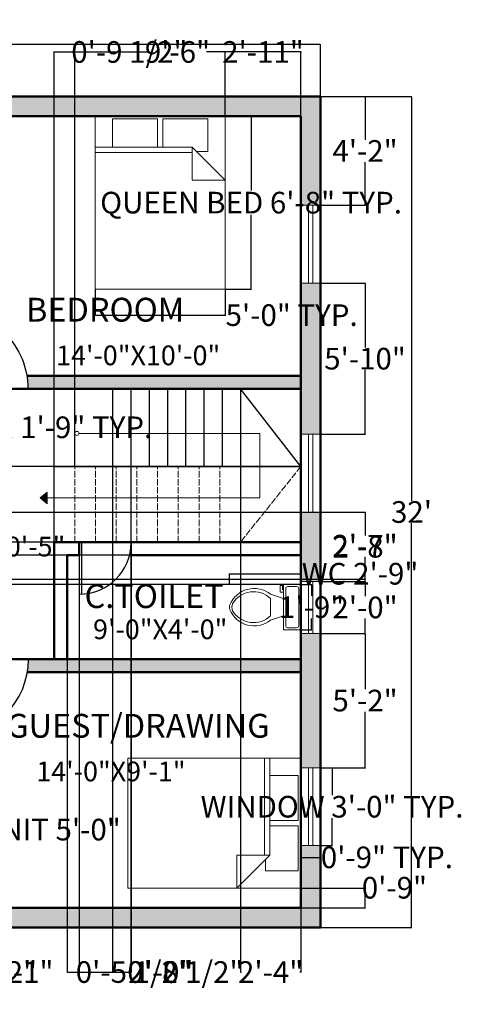
# Model space of a CAD drawing. Units: inches. Extents: x 168 to 640, y -211 to 244.
# Tile 3 of 3: x 436 to 640, y -211 to 244. Entities that reach past the tile are written whole.
import ezdxf

# ---------------------------------------------------------------- set-up
doc = ezdxf.new("R2010")
doc.units = ezdxf.units.IN
doc.header["$MEASUREMENT"] = 0
doc.linetypes.add('ACAD_ISO02W100', pattern=[15, 12, -3])
for name, color, linetype, lineweight in [('A-ANNO-DIMS', 2, 'Continuous', 18), ('A-ANNO-SYMB', 7, 'Continuous', 18), ('A-AREA-IDEN', 7, 'Continuous', 25), ('A-DOOR', 4, 'Continuous', 25), ('A-FLOR-FIXT', 9, 'Continuous', 18), ('A-FLOR-STRS', 7, 'Continuous', 25), ('A-FLOR-STRS-OVHD', 8, 'ACAD_ISO02W100', 18), ('A-FURN', 8, 'Continuous', 18), ('A-GLAZ', 4, 'Continuous', 18), ('A-WALL', 7, 'Continuous', 50)]:
    doc.layers.add(name, color=color, linetype=linetype, lineweight=lineweight)
doc.layers.add('A-WALL-PATT', color=251, linetype='Continuous', lineweight=13, true_color=0x636466)
doc.styles.get("Standard").update_dxf_attribs({"font": 'arial.ttf'})
doc.dimstyles.get("Standard").update_dxf_attribs({"dimtxt": 10, "dimasz": 0.18, "dimexe": 0.18, "dimexo": 0.0625, "dimgap": 0.09, "dimtad": 0, "dimtih": 1, "dimtoh": 1, "dimdec": 0, "dimzin": 0, "dimdsep": 46, "dimlunit": 3, "dimtxsty": 'Standard', "dimcen": 0.09, "dimadec": 0, "dimazin": 0, "dimtfac": 1, "dimtdec": 0, "dimtofl": 0, "dimtmove": 0, "dimatfit": 3, "dimfxl": 1, "dimtolj": 1, "dimtzin": 0, "dimarcsym": 0})

# ---------------------------------------------------------------- blocks, each defined once
blk = doc.blocks.new('*D1')
at = {"layer": 'A-ANNO-DIMS', "color": 0, "lineweight": -2, "transparency": 16777216}
for p, q in [((574.7, 208.8), (616.93, 208.8)), ((616.75, 208.62), (616.75, 22)), ((616.75, -175.02), (616.75, 11.6)), ((574.7, -175.2), (616.93, -175.2))]:
    blk.add_line(p, q, dxfattribs=at)
at = {"layer": 'A-ANNO-DIMS', "color": 0, "transparency": 16777216}
for points in [[(616.72, 208.62), (616.78, 208.62), (616.75, 208.8)], [(616.72, -175.02), (616.78, -175.02), (616.75, -175.2)]]:
    blk.add_solid(points, dxfattribs=at)
at = {"layer": 'Defpoints', "color": 0, "transparency": 16777216}
for p in [(574.63, 208.8), (574.63, -175.2), (616.75, -175.2)]:
    blk.add_point(p, dxfattribs=at)
at = {"layer": 'A-ANNO-DIMS', "color": 0, "transparency": 16777216, "insert": (616.75, 16.8), "char_height": 10, "attachment_point": 5}
blk.add_mtext("\\A1;32'", dxfattribs=at)
blk = doc.blocks.new('*D2')
at = {"layer": 'A-ANNO-DIMS', "color": 0, "lineweight": -2, "transparency": 16777216}
for p, q in [((214.63, 208.86), (214.63, 233.12)), ((214.81, 232.94), (386.06, 232.94)), ((574.45, 232.94), (403.21, 232.94)), ((574.63, 208.86), (574.63, 233.12))]:
    blk.add_line(p, q, dxfattribs=at)
at = {"layer": 'A-ANNO-DIMS', "color": 0, "transparency": 16777216}
for points in [[(214.81, 232.97), (214.81, 232.91), (214.63, 232.94)], [(574.45, 232.97), (574.45, 232.91), (574.63, 232.94)]]:
    blk.add_solid(points, dxfattribs=at)
at = {"layer": 'Defpoints', "color": 0, "transparency": 16777216}
for p in [(214.63, 232.94), (214.63, 208.8), (574.63, 208.8)]:
    blk.add_point(p, dxfattribs=at)
at = {"layer": 'A-ANNO-DIMS', "color": 0, "transparency": 16777216, "insert": (394.63, 232.94), "char_height": 10, "attachment_point": 5}
blk.add_mtext("\\A1;30'", dxfattribs=at)
blk = doc.blocks.new('Toilet - top')
for p, q in [((9.5, -6), (9.5, -2)), ((-10, -8.5), (-8, -8.5)), ((-10, -9.5), (-10, -8.5)), ((-8, -8.5), (-8, -8)), ((-7, -8), (-7, -9.5)), ((-4, -8), (-6, -14)), ((4, -8), (6, -14)), ((-7, -9.5), (-10, -9.5)), ((4, -14), (-4, -14))]:
    blk.add_line(p, q)
blk.add_lwpolyline([(10.5, -8), (10.5, 0), (-10.5, 0), (-10.5, -8)], close=True)
for points in [[(-9.5, -2), (-9.5, -6)], [(8.5, -1), (-8.5, -1)], [(-8.5, -7), (8.5, -7)]]:
    blk.add_lwpolyline(points)
for centre, radius, start, end in [((-8.62, -1.88), 0.884, 81.8699, 188.1301), ((8.62, -1.88), 0.884, 351.8699, 98.1301), ((-8.62, -6.12), 0.884, 171.8699, 278.1301), ((8.62, -6.12), 0.884, 261.8699, 8.1301), ((3.52, -21.58), 12.17, 141.4691, 247.9714), ((4.2, -21.82), 11.33, 136.3677, 238.9468), ((-3.52, -21.58), 12.17, 292.0284, 38.5307), ((-4.2, -21.82), 11.33, 301.053, 43.6321), ((0, -27.88), 4, 245.7318, 294.2682), ((0, -29), 4, 254.8605, 285.1395)]:
    blk.add_arc(centre, radius, start, end)
blk = doc.blocks.new('Bed - Queen')
for p, q in [((0, -80.00003), (0, 0)), ((0, 0), (59.99999, 0)), ((59.99999, 0), (59.99999, -80.00003)), ((7.99999, -1.2), (28.79998, -1.2)), ((7.99999, -14.4), (7.99999, -1.2)), ((28.79998, -1.2), (28.79998, -14.4)), ((31.19999, -1.2), (51.99999, -1.2)), ((31.19999, -14.4), (31.19999, -1.2)), ((51.99999, -1.2), (51.99999, -16.4)), ((0, -14.4), (44.8, -14.4)), ((44.8, -16.8), (0, -16.8)), ((59.99999, -29.6), (44.8, -14.4)), ((44.8, -14.4), (44.8, -29.6)), ((51.99999, -16.4), (46.79936, -16.4)), ((44.8, -29.6), (59.99999, -29.6)), ((59.99999, -80.00003), (0, -80.00003))]:
    blk.add_line(p, q)
blk = doc.blocks.new('DOOR-SWING-36IN')
for p, q in [((0, 36), (0, 0)), ((1, 36), (1, 0))]:
    blk.add_line(p, q)
blk.add_arc((0, 36), 36, 270, 0)
blk = doc.blocks.new('WIN-36IN-WALL9')
at = {"ltscale": 0.25}
for p, q in [((0, 36), (9, 36)), ((3.5, 36), (3.5, 0)), ((5.5, 36), (5.5, 0)), ((9, 0), (0, 0))]:
    blk.add_line(p, q, dxfattribs=at)
blk = doc.blocks.new('*D9')
at = {"layer": 'A-ANNO-DIMS', "color": 0, "lineweight": -2, "ltscale": 0.25, "transparency": 16777216}
for p, q in [((574.7, -101.43), (580.21, -101.43)), ((580.03, -101.61), (580.03, -114.16)), ((580.03, -137.25), (580.03, -124.7)), ((574.7, -137.43), (580.21, -137.43))]:
    blk.add_line(p, q, dxfattribs=at)
at = {"layer": 'A-ANNO-DIMS', "color": 0, "ltscale": 0.25, "transparency": 16777216}
for points in [[(580, -101.61), (580.06, -101.61), (580.03, -101.43)], [(580, -137.25), (580.06, -137.25), (580.03, -137.43)]]:
    blk.add_solid(points, dxfattribs=at)
at = {"layer": 'Defpoints', "color": 0, "ltscale": 0.25, "transparency": 16777216}
for p in [(574.63, -101.43), (580.03, -101.43), (574.63, -137.43)]:
    blk.add_point(p, dxfattribs=at)
at = {"layer": 'A-ANNO-DIMS', "color": 0, "ltscale": 0.25, "transparency": 16777216, "insert": (580.03, -119.43), "char_height": 10, "attachment_point": 5}
blk.add_mtext('\\A1;WINDOW 3\'-0" TYP.', dxfattribs=at)
blk = doc.blocks.new('*D10')
at = {"layer": 'A-ANNO-DIMS', "color": 0, "lineweight": -2, "ltscale": 0.25, "transparency": 16777216}
for p, q in [((565.63, -137.49), (565.63, -143.01)), ((574.63, -137.49), (574.63, -143.01)), ((565.81, -142.83), (574.45, -142.83)), ((574.63, -142.83), (574.81, -142.83))]:
    blk.add_line(p, q, dxfattribs=at)
at = {"layer": 'A-ANNO-DIMS', "color": 0, "ltscale": 0.25, "transparency": 16777216}
for points in [[(565.81, -142.8), (565.81, -142.86), (565.63, -142.83)], [(574.45, -142.8), (574.45, -142.86), (574.63, -142.83)]]:
    blk.add_solid(points, dxfattribs=at)
at = {"layer": 'Defpoints', "color": 0, "ltscale": 0.25, "transparency": 16777216}
for p in [(565.63, -137.43), (574.63, -137.43), (574.63, -142.83)]:
    blk.add_point(p, dxfattribs=at)
at = {"layer": 'A-ANNO-DIMS', "color": 0, "ltscale": 0.25, "transparency": 16777216, "insert": (605.38, -142.83), "char_height": 10, "attachment_point": 5}
blk.add_mtext('\\A1;0\'-9" TYP.', dxfattribs=at)
blk = doc.blocks.new('*D13')
at = {"layer": 'A-ANNO-DIMS', "color": 0, "lineweight": -2, "ltscale": 0.25, "transparency": 16777216}
for p, q in [((530.7, 199.8), (542.82, 199.8)), ((542.64, 199.62), (542.64, 165.37)), ((542.64, 119.98), (542.64, 154.23)), ((530.7, 119.8), (542.82, 119.8))]:
    blk.add_line(p, q, dxfattribs=at)
at = {"layer": 'A-ANNO-DIMS', "color": 0, "ltscale": 0.25, "transparency": 16777216}
for points in [[(542.61, 199.62), (542.67, 199.62), (542.64, 199.8)], [(542.61, 119.98), (542.67, 119.98), (542.64, 119.8)]]:
    blk.add_solid(points, dxfattribs=at)
at = {"layer": 'Defpoints', "color": 0, "ltscale": 0.25, "transparency": 16777216}
for p in [(530.64, 199.8), (542.64, 199.8), (530.64, 119.8)]:
    blk.add_point(p, dxfattribs=at)
at = {"layer": 'A-ANNO-DIMS', "color": 0, "ltscale": 0.25, "transparency": 16777216, "insert": (542.64, 159.8), "char_height": 10, "attachment_point": 5}
blk.add_mtext('\\A1;QUEEN BED 6\'-8" TYP.', dxfattribs=at)
blk = doc.blocks.new('*D14')
at = {"layer": 'A-ANNO-DIMS', "color": 0, "lineweight": -2, "ltscale": 0.25, "transparency": 16777216}
for p, q in [((470.64, 119.74), (470.64, 107.62)), ((530.64, 119.74), (530.64, 107.62)), ((470.82, 107.8), (530.46, 107.8)), ((530.64, 107.8), (530.82, 107.8))]:
    blk.add_line(p, q, dxfattribs=at)
at = {"layer": 'A-ANNO-DIMS', "color": 0, "ltscale": 0.25, "transparency": 16777216}
for points in [[(470.82, 107.83), (470.82, 107.77), (470.64, 107.8)], [(530.46, 107.83), (530.46, 107.77), (530.64, 107.8)]]:
    blk.add_solid(points, dxfattribs=at)
at = {"layer": 'Defpoints', "color": 0, "ltscale": 0.25, "transparency": 16777216}
for p in [(470.64, 119.8), (530.64, 119.8), (530.64, 107.8)]:
    blk.add_point(p, dxfattribs=at)
at = {"layer": 'A-ANNO-DIMS', "color": 0, "ltscale": 0.25, "transparency": 16777216, "insert": (561.38, 107.8), "char_height": 10, "attachment_point": 5}
blk.add_mtext('\\A1;5\'-0" TYP.', dxfattribs=at)
blk = doc.blocks.new('*D15')
at = {"layer": 'A-ANNO-DIMS', "color": 0, "lineweight": -2, "ltscale": 0.25, "transparency": 16777216}
for p, q in [((318.79, 52.86), (318.79, 56.13)), ((318.97, 55.95), (339.61, 55.95)), ((339.79, 52.86), (339.79, 56.13)), ((339.79, 55.95), (339.97, 55.95))]:
    blk.add_line(p, q, dxfattribs=at)
at = {"layer": 'A-ANNO-DIMS', "color": 0, "ltscale": 0.25, "transparency": 16777216}
for points in [[(318.97, 55.98), (318.97, 55.92), (318.79, 55.95)], [(339.61, 55.98), (339.61, 55.92), (339.79, 55.95)]]:
    blk.add_solid(points, dxfattribs=at)
at = {"layer": 'Defpoints', "color": 0, "ltscale": 0.25, "transparency": 16777216}
for p in [(339.79, 55.95), (318.79, 52.8), (339.79, 52.8)]:
    blk.add_point(p, dxfattribs=at)
at = {"layer": 'A-ANNO-DIMS', "color": 0, "ltscale": 0.25, "transparency": 16777216, "insert": (420.35, 55.95), "char_height": 10, "attachment_point": 5}
blk.add_mtext('\\A1;DINING CHAIR 1\'-9" TYP.', dxfattribs=at)
blk = doc.blocks.new('*D17')
at = {"layer": 'A-ANNO-DIMS', "color": 0, "lineweight": -2, "ltscale": 0.25, "transparency": 16777216}
for p, q in [((532.59, -16.64), (532.59, -11.56)), ((532.77, -11.74), (565.45, -11.74)), ((565.63, -16.64), (565.63, -11.56)), ((565.63, -11.74), (565.81, -11.74))]:
    blk.add_line(p, q, dxfattribs=at)
at = {"layer": 'A-ANNO-DIMS', "color": 0, "ltscale": 0.25, "transparency": 16777216}
for points in [[(532.77, -11.71), (532.77, -11.77), (532.59, -11.74)], [(565.45, -11.71), (565.45, -11.77), (565.63, -11.74)]]:
    blk.add_solid(points, dxfattribs=at)
at = {"layer": 'Defpoints', "color": 0, "ltscale": 0.25, "transparency": 16777216}
for p in [(565.63, -11.74), (532.59, -16.7), (565.63, -16.7)]:
    blk.add_point(p, dxfattribs=at)
at = {"layer": 'A-ANNO-DIMS', "color": 0, "ltscale": 0.25, "transparency": 16777216, "insert": (592.98, -11.74), "char_height": 10, "attachment_point": 5}
blk.add_mtext('\\A1;WC 2\'-9"', dxfattribs=at)
blk = doc.blocks.new('*D18')
at = {"layer": 'A-ANNO-DIMS', "color": 0, "lineweight": -2, "ltscale": 0.25, "transparency": 16777216}
for p, q in [((565.7, -16.7), (570.77, -16.7)), ((570.59, -16.88), (570.59, -22)), ((570.59, -37.52), (570.59, -32.4)), ((565.7, -37.7), (570.77, -37.7))]:
    blk.add_line(p, q, dxfattribs=at)
at = {"layer": 'A-ANNO-DIMS', "color": 0, "ltscale": 0.25, "transparency": 16777216}
for points in [[(570.56, -16.88), (570.62, -16.88), (570.59, -16.7)], [(570.56, -37.52), (570.62, -37.52), (570.59, -37.7)]]:
    blk.add_solid(points, dxfattribs=at)
at = {"layer": 'Defpoints', "color": 0, "ltscale": 0.25, "transparency": 16777216}
for p in [(565.63, -16.7), (565.63, -37.7), (570.59, -37.7)]:
    blk.add_point(p, dxfattribs=at)
at = {"layer": 'A-ANNO-DIMS', "color": 0, "ltscale": 0.25, "transparency": 16777216, "insert": (570.59, -27.2), "char_height": 10, "attachment_point": 5}
blk.add_mtext('\\A1;1\'-9"', dxfattribs=at)
blk = doc.blocks.new('*D19')
at = {"layer": 'A-ANNO-DIMS', "color": 0, "lineweight": -2, "ltscale": 0.25, "transparency": 16777216}
for p, q in [((419.03, -100), (428.15, -100)), ((427.97, -100.18), (427.97, -124.81)), ((427.97, -159.82), (427.97, -135.2)), ((419.03, -160), (428.15, -160))]:
    blk.add_line(p, q, dxfattribs=at)
at = {"layer": 'A-ANNO-DIMS', "color": 0, "ltscale": 0.25, "transparency": 16777216}
for points in [[(427.94, -100.18), (428, -100.18), (427.97, -100)], [(427.94, -159.82), (428, -159.82), (427.97, -160)]]:
    blk.add_solid(points, dxfattribs=at)
at = {"layer": 'Defpoints', "color": 0, "ltscale": 0.25, "transparency": 16777216}
for p in [(418.97, -100), (427.97, -100), (418.97, -160)]:
    blk.add_point(p, dxfattribs=at)
at = {"layer": 'A-ANNO-DIMS', "color": 0, "ltscale": 0.25, "transparency": 16777216, "insert": (427.97, -130), "char_height": 10, "attachment_point": 5}
blk.add_mtext('\\A1;MEDIA UNIT 5\'-0"', dxfattribs=at)
blk = doc.blocks.new('*D23')
at = {"layer": 'A-ANNO-DIMS', "color": 0, "lineweight": -2, "ltscale": 0.25, "transparency": 16777216}
for p, q in [((574.7, 208.8), (595.46, 208.8)), ((595.28, 208.62), (595.28, 188.79)), ((595.28, 158.75), (595.28, 178.57)), ((574.7, 158.57), (595.46, 158.57))]:
    blk.add_line(p, q, dxfattribs=at)
at = {"layer": 'A-ANNO-DIMS', "color": 0, "ltscale": 0.25, "transparency": 16777216}
for points in [[(595.25, 208.62), (595.31, 208.62), (595.28, 208.8)], [(595.25, 158.75), (595.31, 158.75), (595.28, 158.57)]]:
    blk.add_solid(points, dxfattribs=at)
at = {"layer": 'Defpoints', "color": 0, "ltscale": 0.25, "transparency": 16777216}
for p in [(574.63, 208.8), (574.63, 158.57), (595.28, 158.57)]:
    blk.add_point(p, dxfattribs=at)
at = {"layer": 'A-ANNO-DIMS', "color": 0, "ltscale": 0.25, "transparency": 16777216, "insert": (595.28, 183.68), "char_height": 10, "attachment_point": 5}
blk.add_mtext('\\A1;4\'-2"', dxfattribs=at)
blk = doc.blocks.new('*D24')
at = {"layer": 'A-ANNO-DIMS', "color": 0, "lineweight": -2, "ltscale": 0.25, "transparency": 16777216}
for p, q in [((574.7, 122.57), (595.46, 122.57)), ((595.28, 122.39), (595.28, 92.88)), ((595.28, 52.98), (595.28, 82.49)), ((574.7, 52.8), (595.46, 52.8))]:
    blk.add_line(p, q, dxfattribs=at)
at = {"layer": 'A-ANNO-DIMS', "color": 0, "ltscale": 0.25, "transparency": 16777216}
for points in [[(595.25, 122.39), (595.31, 122.39), (595.28, 122.57)], [(595.25, 52.98), (595.31, 52.98), (595.28, 52.8)]]:
    blk.add_solid(points, dxfattribs=at)
at = {"layer": 'Defpoints', "color": 0, "ltscale": 0.25, "transparency": 16777216}
for p in [(574.63, 122.57), (574.63, 52.8), (595.28, 52.8)]:
    blk.add_point(p, dxfattribs=at)
at = {"layer": 'A-ANNO-DIMS', "color": 0, "ltscale": 0.25, "transparency": 16777216, "insert": (595.28, 87.68), "char_height": 10, "attachment_point": 5}
blk.add_mtext('\\A1;5\'-10"', dxfattribs=at)
blk = doc.blocks.new('*D25')
at = {"layer": 'A-ANNO-DIMS', "color": 0, "lineweight": -2, "ltscale": 0.25, "transparency": 16777216}
for p, q in [((574.7, 16.8), (595.46, 16.8)), ((595.28, 16.62), (595.28, 5.93)), ((595.28, -15.15), (595.28, -4.46)), ((574.7, -15.33), (595.46, -15.33))]:
    blk.add_line(p, q, dxfattribs=at)
at = {"layer": 'A-ANNO-DIMS', "color": 0, "ltscale": 0.25, "transparency": 16777216}
for points in [[(595.25, 16.62), (595.31, 16.62), (595.28, 16.8)], [(595.25, -15.15), (595.31, -15.15), (595.28, -15.33)]]:
    blk.add_solid(points, dxfattribs=at)
at = {"layer": 'Defpoints', "color": 0, "ltscale": 0.25, "transparency": 16777216}
for p in [(574.63, 16.8), (574.63, -15.33), (595.28, -15.33)]:
    blk.add_point(p, dxfattribs=at)
at = {"layer": 'A-ANNO-DIMS', "color": 0, "ltscale": 0.25, "transparency": 16777216, "insert": (595.28, 0.74), "char_height": 10, "attachment_point": 5}
blk.add_mtext('\\A1;2\'-8"', dxfattribs=at)
blk = doc.blocks.new('*D26')
at = {"layer": 'A-ANNO-DIMS', "color": 0, "lineweight": -2, "ltscale": 0.25, "transparency": 16777216}
for p, q in [((574.7, -15.33), (595.46, -15.33)), ((595.28, -15.51), (595.28, -22.11)), ((595.28, -39.11), (595.28, -32.5)), ((574.7, -39.29), (595.46, -39.29))]:
    blk.add_line(p, q, dxfattribs=at)
at = {"layer": 'A-ANNO-DIMS', "color": 0, "ltscale": 0.25, "transparency": 16777216}
for points in [[(595.25, -15.51), (595.31, -15.51), (595.28, -15.33)], [(595.25, -39.11), (595.31, -39.11), (595.28, -39.29)]]:
    blk.add_solid(points, dxfattribs=at)
at = {"layer": 'Defpoints', "color": 0, "ltscale": 0.25, "transparency": 16777216}
for p in [(574.63, -15.33), (574.63, -39.29), (595.28, -39.29)]:
    blk.add_point(p, dxfattribs=at)
at = {"layer": 'A-ANNO-DIMS', "color": 0, "ltscale": 0.25, "transparency": 16777216, "insert": (595.28, -27.31), "char_height": 10, "attachment_point": 5}
blk.add_mtext('\\A1;2\'-0"', dxfattribs=at)
blk = doc.blocks.new('*D27')
at = {"layer": 'A-ANNO-DIMS', "color": 0, "lineweight": -2, "ltscale": 0.25, "transparency": 16777216}
for p, q in [((574.7, -39.29), (595.46, -39.29)), ((595.28, -39.47), (595.28, -65.16)), ((595.28, -101.25), (595.28, -75.56)), ((574.7, -101.43), (595.46, -101.43))]:
    blk.add_line(p, q, dxfattribs=at)
at = {"layer": 'A-ANNO-DIMS', "color": 0, "ltscale": 0.25, "transparency": 16777216}
for points in [[(595.25, -39.47), (595.31, -39.47), (595.28, -39.29)], [(595.25, -101.25), (595.31, -101.25), (595.28, -101.43)]]:
    blk.add_solid(points, dxfattribs=at)
at = {"layer": 'Defpoints', "color": 0, "ltscale": 0.25, "transparency": 16777216}
for p in [(574.63, -39.29), (574.63, -101.43), (595.28, -101.43)]:
    blk.add_point(p, dxfattribs=at)
at = {"layer": 'A-ANNO-DIMS', "color": 0, "ltscale": 0.25, "transparency": 16777216, "insert": (595.28, -70.36), "char_height": 10, "attachment_point": 5}
blk.add_mtext('\\A1;5\'-2"', dxfattribs=at)
blk = doc.blocks.new('*D32')
at = {"layer": 'A-ANNO-DIMS', "color": 0, "lineweight": -2, "ltscale": 0.25, "transparency": 16777216}
for p, q in [((451.63, 2.86), (451.63, 229.63)), ((451.81, 229.45), (495.25, 229.45)), ((565.45, 229.45), (522.02, 229.45)), ((565.63, 2.86), (565.63, 229.63))]:
    blk.add_line(p, q, dxfattribs=at)
at = {"layer": 'A-ANNO-DIMS', "color": 0, "ltscale": 0.25, "transparency": 16777216}
for points in [[(451.81, 229.48), (451.81, 229.42), (451.63, 229.45)], [(565.45, 229.48), (565.45, 229.42), (565.63, 229.45)]]:
    blk.add_solid(points, dxfattribs=at)
at = {"layer": 'Defpoints', "color": 0, "ltscale": 0.25, "transparency": 16777216}
for p in [(565.63, 229.45), (451.63, 2.8), (565.63, 2.8)]:
    blk.add_point(p, dxfattribs=at)
at = {"layer": 'A-ANNO-DIMS', "color": 0, "ltscale": 0.25, "transparency": 16777216, "insert": (508.63, 229.45), "char_height": 10, "attachment_point": 5}
blk.add_mtext('\\A1;9\'-6"', dxfattribs=at)
blk = doc.blocks.new('*D33')
at = {"layer": 'A-ANNO-DIMS', "color": 0, "lineweight": -2, "ltscale": 0.25, "transparency": 16777216}
for p, q in [((565.57, 73.8), (193.8, 73.8)), ((193.98, 73.62), (193.98, 61)), ((193.98, 37.98), (193.98, 50.6)), ((565.57, 37.8), (193.8, 37.8))]:
    blk.add_line(p, q, dxfattribs=at)
at = {"layer": 'A-ANNO-DIMS', "color": 0, "ltscale": 0.25, "transparency": 16777216}
for points in [[(193.95, 73.62), (194.01, 73.62), (193.98, 73.8)], [(193.95, 37.98), (194.01, 37.98), (193.98, 37.8)]]:
    blk.add_solid(points, dxfattribs=at)
at = {"layer": 'Defpoints', "color": 0, "ltscale": 0.25, "transparency": 16777216}
for p in [(193.98, 73.8), (565.63, 73.8), (565.63, 37.8)]:
    blk.add_point(p, dxfattribs=at)
at = {"layer": 'A-ANNO-DIMS', "color": 0, "ltscale": 0.25, "transparency": 16777216, "insert": (193.98, 55.8), "char_height": 10, "attachment_point": 5}
blk.add_mtext('\\A1;3\'-0"', dxfattribs=at)
blk = doc.blocks.new('*D34')
at = {"layer": 'A-ANNO-DIMS', "color": 0, "lineweight": -2, "ltscale": 0.25, "transparency": 16777216}
for p, q in [((451.57, 37.8), (193.8, 37.8)), ((193.98, 37.62), (193.98, 25.41)), ((193.98, 2.98), (193.98, 15.19)), ((451.57, 2.8), (193.8, 2.8))]:
    blk.add_line(p, q, dxfattribs=at)
at = {"layer": 'A-ANNO-DIMS', "color": 0, "ltscale": 0.25, "transparency": 16777216}
for points in [[(193.95, 37.62), (194.01, 37.62), (193.98, 37.8)], [(193.95, 2.98), (194.01, 2.98), (193.98, 2.8)]]:
    blk.add_solid(points, dxfattribs=at)
at = {"layer": 'Defpoints', "color": 0, "ltscale": 0.25, "transparency": 16777216}
for p in [(193.98, 37.8), (451.63, 37.8), (451.63, 2.8)]:
    blk.add_point(p, dxfattribs=at)
at = {"layer": 'A-ANNO-DIMS', "color": 0, "ltscale": 0.25, "transparency": 16777216, "insert": (193.98, 20.3), "char_height": 10, "attachment_point": 5}
blk.add_mtext('\\A1;2\'-11"', dxfattribs=at)
blk = doc.blocks.new('*D40')
at = {"layer": 'A-ANNO-DIMS', "color": 0, "lineweight": -2, "ltscale": 0.25, "transparency": 16777216}
for p, q in [((457.63, -3.26), (457.63, -196.03)), ((463.26, -3.26), (463.26, -196.03)), ((457.81, -195.85), (463.08, -195.85)), ((463.26, -195.85), (463.44, -195.85))]:
    blk.add_line(p, q, dxfattribs=at)
at = {"layer": 'A-ANNO-DIMS', "color": 0, "ltscale": 0.25, "transparency": 16777216}
for points in [[(457.81, -195.82), (457.81, -195.88), (457.63, -195.85)], [(463.08, -195.82), (463.08, -195.88), (463.26, -195.85)]]:
    blk.add_solid(points, dxfattribs=at)
at = {"layer": 'Defpoints', "color": 0, "ltscale": 0.25, "transparency": 16777216}
for p in [(457.63, -3.2), (463.26, -3.2), (463.26, -195.85)]:
    blk.add_point(p, dxfattribs=at)
at = {"layer": 'A-ANNO-DIMS', "color": 0, "ltscale": 0.25, "transparency": 16777216, "insert": (488.48, -195.85), "char_height": 10, "attachment_point": 5}
blk.add_mtext('\\A1;0\'-5 1/2"', dxfattribs=at)
blk = doc.blocks.new('*D41')
at = {"layer": 'A-ANNO-DIMS', "color": 0, "lineweight": -2, "ltscale": 0.25, "transparency": 16777216}
for p, q in [((463.26, 2.74), (463.26, -196.03)), ((487.26, 2.74), (487.26, -196.03)), ((463.44, -195.85), (487.08, -195.85)), ((487.26, -195.85), (487.44, -195.85))]:
    blk.add_line(p, q, dxfattribs=at)
at = {"layer": 'A-ANNO-DIMS', "color": 0, "ltscale": 0.25, "transparency": 16777216}
for points in [[(463.44, -195.82), (463.44, -195.88), (463.26, -195.85)], [(487.08, -195.82), (487.08, -195.88), (487.26, -195.85)]]:
    blk.add_solid(points, dxfattribs=at)
at = {"layer": 'Defpoints', "color": 0, "ltscale": 0.25, "transparency": 16777216}
for p in [(463.26, 2.8), (487.26, 2.8), (487.26, -195.85)]:
    blk.add_point(p, dxfattribs=at)
at = {"layer": 'A-ANNO-DIMS', "color": 0, "ltscale": 0.25, "transparency": 16777216, "insert": (500.91, -195.85), "char_height": 10, "attachment_point": 5}
blk.add_mtext('\\A1;2\'-0"', dxfattribs=at)
blk = doc.blocks.new('*D42')
at = {"layer": 'A-ANNO-DIMS', "color": 0, "lineweight": -2, "ltscale": 0.25, "transparency": 16777216}
for p, q in [((537.7, 37.74), (537.7, -196.03)), ((565.63, 37.74), (565.63, -196.03)), ((537.88, -195.85), (538.2, -195.85)), ((565.45, -195.85), (565.14, -195.85))]:
    blk.add_line(p, q, dxfattribs=at)
at = {"layer": 'A-ANNO-DIMS', "color": 0, "ltscale": 0.25, "transparency": 16777216}
for points in [[(537.88, -195.82), (537.88, -195.88), (537.7, -195.85)], [(565.45, -195.82), (565.45, -195.88), (565.63, -195.85)]]:
    blk.add_solid(points, dxfattribs=at)
at = {"layer": 'Defpoints', "color": 0, "ltscale": 0.25, "transparency": 16777216}
for p in [(537.7, 37.8), (565.63, 37.8), (565.63, -195.85)]:
    blk.add_point(p, dxfattribs=at)
at = {"layer": 'A-ANNO-DIMS', "color": 0, "ltscale": 0.25, "transparency": 16777216, "insert": (551.67, -195.85), "char_height": 10, "attachment_point": 5}
blk.add_mtext('\\A1;2\'-4"', dxfattribs=at)
blk = doc.blocks.new('*D43')
at = {"layer": 'A-ANNO-DIMS', "color": 0, "lineweight": -2, "ltscale": 0.25, "transparency": 16777216}
for p, q in [((478.63, 73.74), (478.63, -196.03)), ((487.07, 73.74), (487.07, -196.03)), ((478.81, -195.85), (486.89, -195.85)), ((487.07, -195.85), (487.25, -195.85))]:
    blk.add_line(p, q, dxfattribs=at)
at = {"layer": 'A-ANNO-DIMS', "color": 0, "ltscale": 0.25, "transparency": 16777216}
for points in [[(478.81, -195.82), (478.81, -195.88), (478.63, -195.85)], [(486.89, -195.82), (486.89, -195.88), (487.07, -195.85)]]:
    blk.add_solid(points, dxfattribs=at)
at = {"layer": 'Defpoints', "color": 0, "ltscale": 0.25, "transparency": 16777216}
for p in [(478.63, 73.8), (487.07, 73.8), (487.07, -195.85)]:
    blk.add_point(p, dxfattribs=at)
at = {"layer": 'A-ANNO-DIMS', "color": 0, "ltscale": 0.25, "transparency": 16777216, "insert": (512.28, -195.85), "char_height": 10, "attachment_point": 5}
blk.add_mtext('\\A1;0\'-8 1/2"', dxfattribs=at)
blk = doc.blocks.new('*D44')
at = {"layer": 'A-ANNO-DIMS', "color": 0, "lineweight": -2, "ltscale": 0.25, "transparency": 16777216}
for p, q in [((451.63, 37.86), (451.63, 229.63)), ((451.81, 229.45), (461.02, 229.45)), ((461.2, 37.86), (461.2, 229.63)), ((461.2, 229.45), (461.38, 229.45))]:
    blk.add_line(p, q, dxfattribs=at)
at = {"layer": 'A-ANNO-DIMS', "color": 0, "ltscale": 0.25, "transparency": 16777216}
for points in [[(451.81, 229.48), (451.81, 229.42), (451.63, 229.45)], [(461.02, 229.48), (461.02, 229.42), (461.2, 229.45)]]:
    blk.add_solid(points, dxfattribs=at)
at = {"layer": 'Defpoints', "color": 0, "ltscale": 0.25, "transparency": 16777216}
for p in [(461.2, 229.45), (451.63, 37.8), (461.2, 37.8)]:
    blk.add_point(p, dxfattribs=at)
at = {"layer": 'A-ANNO-DIMS', "color": 0, "ltscale": 0.25, "transparency": 16777216, "insert": (486.41, 229.45), "char_height": 10, "attachment_point": 5}
blk.add_mtext('\\A1;0\'-9 1/2"', dxfattribs=at)
blk = doc.blocks.new('*D49')
at = {"layer": 'A-ANNO-DIMS', "color": 0, "lineweight": -2, "ltscale": 0.25, "transparency": 16777216}
for p, q in [((252.23, 16.8), (595.46, 16.8)), ((595.28, 16.62), (595.28, 6.35)), ((595.28, -14.14), (595.28, -3.87)), ((252.23, -14.32), (595.46, -14.32))]:
    blk.add_line(p, q, dxfattribs=at)
at = {"layer": 'A-ANNO-DIMS', "color": 0, "ltscale": 0.25, "transparency": 16777216}
for points in [[(595.25, 16.62), (595.31, 16.62), (595.28, 16.8)], [(595.25, -14.14), (595.31, -14.14), (595.28, -14.32)]]:
    blk.add_solid(points, dxfattribs=at)
at = {"layer": 'Defpoints', "color": 0, "ltscale": 0.25, "transparency": 16777216}
for p in [(252.17, 16.8), (595.28, 16.8), (252.17, -14.32)]:
    blk.add_point(p, dxfattribs=at)
at = {"layer": 'A-ANNO-DIMS', "color": 0, "ltscale": 0.25, "transparency": 16777216, "insert": (595.28, 1.24), "char_height": 10, "attachment_point": 5}
blk.add_mtext('\\A1;2\'-7"', dxfattribs=at)
blk = doc.blocks.new('*D53')
at = {"layer": 'A-ANNO-DIMS', "color": 0, "lineweight": -2, "ltscale": 0.25, "transparency": 16777216}
for p, q in [((367.04, 124.86), (367.04, -196.03)), ((391.63, 124.86), (391.63, -196.03)), ((367.22, -195.85), (391.45, -195.85)), ((391.63, -195.85), (391.81, -195.85))]:
    blk.add_line(p, q, dxfattribs=at)
at = {"layer": 'A-ANNO-DIMS', "color": 0, "ltscale": 0.25, "transparency": 16777216}
for points in [[(367.22, -195.82), (367.22, -195.88), (367.04, -195.85)], [(391.45, -195.82), (391.45, -195.88), (391.63, -195.85)]]:
    blk.add_solid(points, dxfattribs=at)
at = {"layer": 'Defpoints', "color": 0, "ltscale": 0.25, "transparency": 16777216}
for p in [(367.04, 124.92), (391.63, 124.92), (391.63, -195.85)]:
    blk.add_point(p, dxfattribs=at)
at = {"layer": 'A-ANNO-DIMS', "color": 0, "ltscale": 0.25, "transparency": 16777216, "insert": (416.93, -195.85), "char_height": 10, "attachment_point": 5}
blk.add_mtext('\\A1;2\'-0 1/2"', dxfattribs=at)
blk = doc.blocks.new('*D55')
at = {"layer": 'A-ANNO-DIMS', "color": 0, "lineweight": -2, "ltscale": 0.25, "transparency": 16777216}
for p, q in [((397.63, 124.86), (397.63, -196.03)), ((422.63, 124.86), (422.63, -196.03)), ((397.81, -195.85), (422.45, -195.85)), ((422.63, -195.85), (422.81, -195.85))]:
    blk.add_line(p, q, dxfattribs=at)
at = {"layer": 'A-ANNO-DIMS', "color": 0, "ltscale": 0.25, "transparency": 16777216}
for points in [[(397.81, -195.82), (397.81, -195.88), (397.63, -195.85)], [(422.45, -195.82), (422.45, -195.88), (422.63, -195.85)]]:
    blk.add_solid(points, dxfattribs=at)
at = {"layer": 'Defpoints', "color": 0, "ltscale": 0.25, "transparency": 16777216}
for p in [(397.63, 124.92), (422.63, 124.92), (422.63, -195.85)]:
    blk.add_point(p, dxfattribs=at)
at = {"layer": 'A-ANNO-DIMS', "color": 0, "ltscale": 0.25, "transparency": 16777216, "insert": (436.28, -195.85), "char_height": 10, "attachment_point": 5}
blk.add_mtext('\\A1;2\'-1"', dxfattribs=at)
blk = doc.blocks.new('*D57')
at = {"layer": 'A-ANNO-DIMS', "color": 0, "lineweight": -2, "ltscale": 0.25, "transparency": 16777216}
for p, q in [((530.46, 229.45), (530.28, 229.45)), ((530.64, 199.86), (530.64, 229.63)), ((565.63, 199.86), (565.63, 229.63)), ((565.81, 229.45), (565.99, 229.45))]:
    blk.add_line(p, q, dxfattribs=at)
at = {"layer": 'A-ANNO-DIMS', "color": 0, "ltscale": 0.25, "transparency": 16777216}
for points in [[(530.46, 229.48), (530.46, 229.42), (530.64, 229.45)], [(565.81, 229.48), (565.81, 229.42), (565.63, 229.45)]]:
    blk.add_solid(points, dxfattribs=at)
at = {"layer": 'Defpoints', "color": 0, "ltscale": 0.25, "transparency": 16777216}
for p in [(565.63, 229.45), (530.64, 199.8), (565.63, 199.8)]:
    blk.add_point(p, dxfattribs=at)
at = {"layer": 'A-ANNO-DIMS', "color": 0, "ltscale": 0.25, "transparency": 16777216, "insert": (548.14, 229.45), "char_height": 10, "attachment_point": 5}
blk.add_mtext('\\A1;2\'-11"', dxfattribs=at)
blk = doc.blocks.new('*D58')
at = {"layer": 'A-ANNO-DIMS', "color": 0, "lineweight": -2, "ltscale": 0.25, "transparency": 16777216}
for p, q in [((565.7, -157.06), (595.46, -157.06)), ((595.28, -157.06), (595.28, -156.88)), ((595.28, -156.88), (595.46, -156.88)), ((595.28, -166.02), (595.28, -157.24)), ((565.7, -166.2), (595.46, -166.2))]:
    blk.add_line(p, q, dxfattribs=at)
at = {"layer": 'A-ANNO-DIMS', "color": 0, "ltscale": 0.25, "transparency": 16777216}
for points in [[(595.25, -157.24), (595.31, -157.24), (595.28, -157.06)], [(595.25, -166.02), (595.31, -166.02), (595.28, -166.2)]]:
    blk.add_solid(points, dxfattribs=at)
at = {"layer": 'Defpoints', "color": 0, "ltscale": 0.25, "transparency": 16777216}
for p in [(565.63, -157.06), (595.28, -157.06), (565.63, -166.2)]:
    blk.add_point(p, dxfattribs=at)
at = {"layer": 'A-ANNO-DIMS', "color": 0, "ltscale": 0.25, "transparency": 16777216, "insert": (608.85, -156.88), "char_height": 10, "attachment_point": 5}
blk.add_mtext('\\A1;0\'-9"', dxfattribs=at)
blk = doc.blocks.new('*D62')
at = {"layer": 'A-ANNO-DIMS', "color": 0, "lineweight": -2, "ltscale": 0.25, "transparency": 16777216}
for p, q in [((565.57, -3.2), (193.8, -3.2)), ((193.98, -3.38), (193.98, -4.69)), ((565.57, -16.7), (193.8, -16.7)), ((193.98, -16.52), (193.98, -15.21))]:
    blk.add_line(p, q, dxfattribs=at)
at = {"layer": 'A-ANNO-DIMS', "color": 0, "ltscale": 0.25, "transparency": 16777216}
for points in [[(193.95, -3.38), (194.01, -3.38), (193.98, -3.2)], [(193.95, -16.52), (194.01, -16.52), (193.98, -16.7)]]:
    blk.add_solid(points, dxfattribs=at)
at = {"layer": 'Defpoints', "color": 0, "ltscale": 0.25, "transparency": 16777216}
for p in [(565.63, -3.2), (193.98, -16.7), (565.63, -16.7)]:
    blk.add_point(p, dxfattribs=at)
at = {"layer": 'A-ANNO-DIMS', "color": 0, "ltscale": 0.25, "transparency": 16777216, "insert": (193.98, -9.95), "char_height": 10, "attachment_point": 5}
blk.add_mtext('\\A1;1\'-1 1/2"', dxfattribs=at)

msp = doc.modelspace()

# ---------------------------------------------------------------- hatches: boundary and pattern name
at = {"layer": 'A-ANNO-SYMB', "ltscale": 0.25}
h = msp.add_hatch(color=256, dxfattribs=at)
h.dxf.hatch_style = 1
h.paths.add_polyline_path([(448.5, 26.03), (445.23, 23.32), (448.5, 23.32)])
h.paths.add_polyline_path([(448.5, 23.32), (445.23, 23.32), (448.5, 20.61)])
at = {"layer": 'A-WALL-PATT', "ltscale": 0.25}
h = msp.add_hatch(color=256, dxfattribs=at)
h.dxf.hatch_style = 1
h.paths.add_polyline_path([(223.63, 11.3), (214.63, 11.3), (214.63, -175.2), (574.63, -175.2), (574.63, -137.43), (565.63, -137.43), (565.63, -157.06), (565.63, -166.2), (223.63, -166.2)])
h.paths.add_polyline_path([(349.62, -51.2), (301.63, -51.2), (223.63, -51.2), (223.63, -57.2), (301.63, -57.2), (349.12, -57.2, -0.041886)], flags=17)
h.paths.add_polyline_path([(301.63, -48.03), (295.63, -48.03), (295.63, -51.2), (301.63, -51.2)], flags=17)
h.paths.add_polyline_path([(403.8, -51.2), (385.12, -51.2), (385.12, -57.2), (403.8, -57.2)], flags=17)
h.paths.add_polyline_path([(397.63, -57.2), (390.63, -57.2), (390.63, -166.2), (397.63, -166.2)], flags=17)
h.paths.add_polyline_path([(301.63, 73.8), (295.63, 73.8), (295.63, -12.53, -0.041886), (301.63, -12.03)])
h.paths.add_polyline_path([(223.63, 122.57), (214.63, 122.57), (214.63, 47.3), (223.63, 47.3), (223.63, 73.8)])
h.paths.add_polyline_path([(350.92, 79.8), (223.63, 79.8), (223.63, 73.8), (350.42, 73.8, -0.041886)])
h.paths.add_polyline_path([(574.63, 208.8), (214.63, 208.8), (214.63, 158.57), (223.63, 158.57), (223.63, 199.8), (565.63, 199.8), (565.63, 158.57), (574.63, 158.57)])
h.paths.add_polyline_path([(397.63, 199.8), (391.63, 199.8), (391.63, 79.8), (386.42, 79.8), (386.42, 73.8), (391.63, 73.8), (403.56, 73.8), (403.56, 79.8), (397.63, 79.8)])
h.paths.add_polyline_path([(565.63, 79.8), (439.06, 79.8, -0.041886), (439.56, 73.8), (565.63, 73.8)])
h.paths.add_polyline_path([(574.63, 122.57), (565.63, 122.57), (565.63, 79.8), (565.63, 52.8), (574.63, 52.8)])
h.paths.add_polyline_path([(574.63, 16.8), (565.63, 16.8), (565.63, -15.33), (574.63, -15.33)])
h.paths.add_polyline_path([(574.63, -39.29), (570.13, -39.29), (565.63, -39.29), (565.63, -51.2), (565.63, -101.43), (574.63, -101.43)], flags=17)
h.paths.add_polyline_path([(565.63, -51.2), (439.8, -51.2, -0.041886), (439.3, -57.2), (565.63, -57.2)], flags=17)

# ---------------------------------------------------------------- linework, layer by layer
at = {"layer": 'A-ANNO-SYMB', "ltscale": 0.25}
for p, q in [((546.69, 53.12), (463.14, 53.12)), ((546.69, 23.32), (546.69, 53.12)), ((445.23, 23.32), (448.5, 26.03)), ((445.23, 23.32), (546.69, 23.32)), ((445.23, 23.32), (448.5, 20.61)), ((448.5, 26.03), (448.5, 20.61))]:
    msp.add_line(p, q, dxfattribs=at)
msp.add_circle((462.2, 53.12), 0.934, dxfattribs=at)
at = {"layer": 'A-DOOR', "ltscale": 0.25}
for p, q in [((464.26, 2.8), (463.26, 2.8)), ((463.26, 2.8), (463.26, -21.2)), ((464.26, 2.8), (464.26, -21.2))]:
    msp.add_line(p, q, dxfattribs=at)
msp.add_arc((463.26, 2.8), 24, 270, 0, dxfattribs=at)
at = {"layer": 'A-FLOR-STRS'}
for p, q in [((478.63, 73.8), (478.63, 37.8)), ((487.07, 73.8), (487.07, 37.8)), ((495.51, 73.8), (495.51, 37.8)), ((503.95, 73.8), (503.95, 37.8)), ((512.39, 73.8), (512.39, 37.8)), ((520.83, 73.8), (520.83, 37.8)), ((529.26, 73.8), (529.26, 37.8)), ((537.7, 73.8), (537.7, 37.8)), ((537.7, 73.8), (537.7, 37.8)), ((451.63, 37.8), (478.63, 37.8)), ((478.63, 37.8), (565.63, 37.8))]:
    msp.add_line(p, q, dxfattribs=at)
at = {"layer": 'A-FLOR-STRS', "ltscale": 0.25}
msp.add_line((565.63, 37.8), (537.7, 73.8), dxfattribs=at)
at = {"layer": 'A-FLOR-STRS-OVHD', "ltscale": 0.25}
for p, q in [((451.63, 2.8), (451.63, 37.8)), ((461.2, 2.8), (461.2, 37.8)), ((470.76, 2.8), (470.76, 37.8)), ((480.32, 2.8), (480.32, 37.8)), ((489.89, 2.8), (489.89, 37.8)), ((499.45, 2.8), (499.45, 37.8)), ((509.01, 2.8), (509.01, 37.8)), ((518.58, 2.8), (518.58, 37.8)), ((528.14, 2.8), (528.14, 37.8)), ((537.7, 2.8), (537.7, 37.8)), ((565.63, 37.8), (537.7, 2.8))]:
    msp.add_line(p, q, dxfattribs=at)
at = {"layer": 'A-GLAZ', "ltscale": 0.25}
for p, q in [((565.63, -15.33), (574.63, -15.33)), ((569.13, -15.33), (569.13, -39.29)), ((571.13, -15.33), (571.13, -39.29)), ((570.13, -39.29), (565.63, -39.29)), ((570.13, -39.29), (574.63, -39.29))]:
    msp.add_line(p, q, dxfattribs=at)
at = {"layer": 'A-WALL'}
for p, q in [((214.63, 208.8), (574.63, 208.8)), ((574.63, -175.2), (574.63, 208.8)), ((223.63, 199.8), (565.63, 199.8)), ((565.63, -166.2), (565.63, 199.8)), ((565.63, 199.8), (565.63, 79.8)), ((565.63, 79.8), (439.06, 79.8)), ((565.63, 73.8), (391.63, 73.8)), ((565.63, 2.8), (451.63, 2.8)), ((451.63, 2.8), (451.63, -51.2)), ((463.26, -3.2), (463.26, 2.8)), ((457.63, -3.2), (457.63, -51.2)), ((463.26, -3.2), (457.63, -3.2)), ((565.63, -3.2), (486.5, -3.2)), ((565.63, -51.2), (565.63, -3.2)), ((565.63, -51.2), (385.12, -51.2)), ((565.63, -57.2), (439.3, -57.2)), ((565.63, -166.2), (565.63, -57.2)), ((223.63, -166.2), (565.63, -166.2)), ((214.63, -175.2), (574.63, -175.2))]:
    msp.add_line(p, q, dxfattribs=at)

# ---------------------------------------------------------------- block references
at = {"layer": 'A-DOOR', "extrusion": (0, 0, -1), "zscale": -1, "rotation": 180}
msp.add_blockref('DOOR-SWING-36IN', (-403.56, 109.8), dxfattribs=at)
at = {"layer": 'A-DOOR'}
msp.add_blockref('DOOR-SWING-36IN', (403.8, -87.2), dxfattribs=at)
at = {"layer": 'A-FLOR-FIXT', "ltscale": 0.25, "rotation": 270}
msp.add_blockref('Toilet - top', (565.63, -27.2), dxfattribs=at)
at = {"layer": 'A-FURN', "ltscale": 0.25}
msp.add_blockref('Bed - Queen', (470.64, 199.8), dxfattribs=at)
at = {"layer": 'A-FURN', "ltscale": 0.25, "rotation": 270}
msp.add_blockref('Bed - Queen', (565.63, -97.06), dxfattribs=at)
at = {"layer": 'A-GLAZ'}
for p in [(565.63, 122.57), (565.63, 16.8), (565.63, -137.43)]:
    msp.add_blockref('WIN-36IN-WALL9', p, dxfattribs=at)

# ---------------------------------------------------------------- texts
at = {"layer": 'A-AREA-IDEN', "ltscale": 0.25}
for s, height, p in [('BEDROOM', 11.012, (438.65, 104.8)), ('14\'-0"X10\'-0"', 9.1115, (452.57, 84.64)), ('12\'-6\'X10\'-5"', 9.1115, (383.42, -3.75)), ('C.TOILET    ', 11.0125, (465.69, -27.59)), ('9\'-0"X4\'-0"', 9.1115, (469.64, -41.99)), ('GUEST/DRAWING', 11.0125, (429.5, -87.52)), ('14\'-0"X9\'-1"', 9.1115, (443.43, -107.68))]:
    msp.add_text(s, height=height, dxfattribs=at).set_placement(p)

# ---------------------------------------------------------------- dimensions: what is measured, and where the dimension line sits
at = {"layer": 'A-ANNO-DIMS', "ltscale": 0.25}
for base, p1, p2, picture, middle in [((461.2, 229.45), (451.63, 37.8), (461.2, 37.8), '*D44', (486.41, 229.45)), ((565.63, 229.45), (451.63, 2.8), (565.63, 2.8), '*D32', (508.63, 229.45)), ((565.63, 229.45), (530.64, 199.8), (565.63, 199.8), '*D57', (548.14, 229.45)), ((391.63, -195.85), (367.04, 124.92), (391.63, 124.92), '*D53', (416.93, -195.85)), ((422.63, -195.85), (397.63, 124.92), (422.63, 124.92), '*D55', (436.28, -195.85)), ((487.07, -195.85), (478.63, 73.8), (487.07, 73.8), '*D43', (512.28, -195.85)), ((565.63, -195.85), (537.7, 37.8), (565.63, 37.8), '*D42', (551.67, -195.85)), ((487.26, -195.85), (463.26, 2.8), (487.26, 2.8), '*D41', (500.91, -195.85)), ((463.26, -195.85), (457.63, -3.2), (463.26, -3.2), '*D40', (488.48, -195.85))]:
    dim = msp.add_linear_dim(base=base, p1=p1, p2=p2, dimstyle='Standard', override={"dimdec": 1, "dimlfac": 1, "dimrnd": 0, "dimzin": 1, "dimdsep": 46, "dimlunit": 4, "dimfrac": 2}, dxfattribs=at)
    dim.commit()
    dim.dimension.update_dxf_attribs({"geometry": picture, "text_midpoint": middle})
at = {"layer": 'A-ANNO-DIMS'}
dim = msp.add_linear_dim(base=(214.63, 232.94), p1=(574.63, 208.8), p2=(214.63, 208.8), dimstyle='Standard', override={"dimclrd": 0, "dimclre": 0, "dimclrt": 0}, dxfattribs=at)
dim.commit()
dim.dimension.update_dxf_attribs({"geometry": '*D2', "text_midpoint": (394.63, 232.94)})
dim = msp.add_linear_dim(base=(616.75, -175.2), p1=(574.63, 208.8), p2=(574.63, -175.2), angle=90, dimstyle='Standard', override={"dimclrd": 0, "dimclre": 0, "dimclrt": 0}, dxfattribs=at)
dim.commit()
dim.dimension.update_dxf_attribs({"geometry": '*D1', "text_midpoint": (616.75, 16.8)})
at = {"layer": 'A-ANNO-DIMS', "ltscale": 0.25}
for base, p1, p2, angle, picture, middle in [((595.28, 158.57), (574.63, 208.8), (574.63, 158.57), 90, '*D23', (595.28, 183.68)), ((595.28, 52.8), (574.63, 122.57), (574.63, 52.8), 90, '*D24', (595.28, 87.68)), ((193.98, 73.8), (565.63, 37.8), (565.63, 73.8), 90, '*D33', (193.98, 55.8)), ((193.98, 37.8), (451.63, 2.8), (451.63, 37.8), 90, '*D34', (193.98, 20.3)), ((595.28, 16.8), (252.17, -14.32), (252.17, 16.8), 90, '*D49', (595.28, 1.24)), ((595.28, -15.33), (574.63, 16.8), (574.63, -15.33), 90, '*D25', (595.28, 0.74)), ((193.98, -16.7), (565.63, -3.2), (565.63, -16.7), 90, '*D62', (193.98, -9.95)), ((570.59, -37.7), (565.63, -16.7), (565.63, -37.7), 270, '*D18', (570.59, -27.2)), ((595.28, -39.29), (574.63, -15.33), (574.63, -39.29), 90, '*D26', (595.28, -27.31)), ((595.28, -101.43), (574.63, -39.29), (574.63, -101.43), 90, '*D27', (595.28, -70.36)), ((595.28, -157.06), (565.63, -166.2), (565.63, -157.06), 90, '*D58', (608.85, -156.88))]:
    dim = msp.add_linear_dim(base=base, p1=p1, p2=p2, angle=angle, dimstyle='Standard', override={"dimdec": 1, "dimlfac": 1, "dimrnd": 0, "dimzin": 1, "dimdsep": 46, "dimlunit": 4, "dimfrac": 2}, dxfattribs=at)
    dim.commit()
    dim.dimension.update_dxf_attribs({"geometry": picture, "text_midpoint": middle})
for base, p1, p2, text, picture, middle in [((542.64, 199.8), (530.64, 119.8), (530.64, 199.8), 'QUEEN BED <> TYP.', '*D13', (542.64, 159.8)), ((427.97, -100), (418.97, -160), (418.97, -100), 'MEDIA UNIT <>', '*D19', (427.97, -130)), ((580.03, -101.43), (574.63, -137.43), (574.63, -101.43), 'WINDOW <> TYP.', '*D9', (580.03, -119.43))]:
    dim = msp.add_linear_dim(base=base, p1=p1, p2=p2, angle=90, text=text, dimstyle='Standard', override={"dimdec": 1, "dimlfac": 1, "dimrnd": 0, "dimzin": 1, "dimdsep": 46, "dimlunit": 4, "dimfrac": 2}, dxfattribs=at)
    dim.commit()
    dim.dimension.update_dxf_attribs({"geometry": picture, "text_midpoint": middle})
for base, p1, p2, text, picture, middle in [((530.64, 107.8), (470.64, 119.8), (530.64, 119.8), '<> TYP.', '*D14', (561.38, 107.8)), ((339.79, 55.95), (318.79, 52.8), (339.79, 52.8), 'DINING CHAIR <> TYP.', '*D15', (420.35, 55.95)), ((565.63, -11.74), (532.59, -16.7), (565.63, -16.7), 'WC <>', '*D17', (592.98, -11.74)), ((574.63, -142.83), (565.63, -137.43), (574.63, -137.43), '<> TYP.', '*D10', (605.38, -142.83))]:
    dim = msp.add_linear_dim(base=base, p1=p1, p2=p2, text=text, dimstyle='Standard', override={"dimdec": 1, "dimlfac": 1, "dimrnd": 0, "dimzin": 1, "dimdsep": 46, "dimlunit": 4, "dimfrac": 2}, dxfattribs=at)
    dim.commit()
    dim.dimension.update_dxf_attribs({"geometry": picture, "text_midpoint": middle})

doc.saveas('drawing.dxf')
